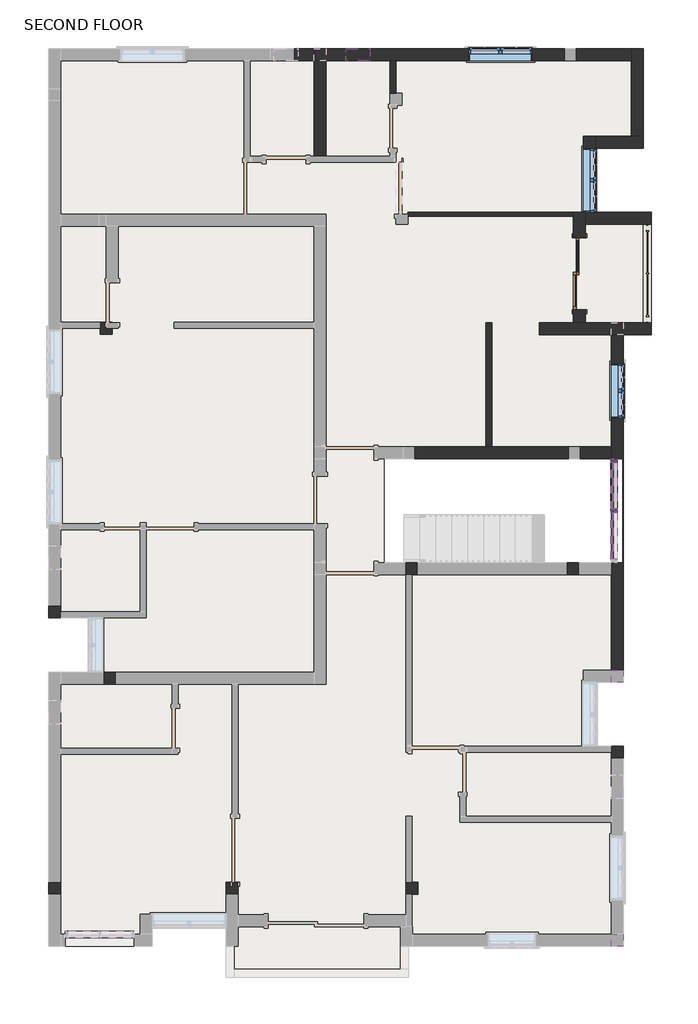
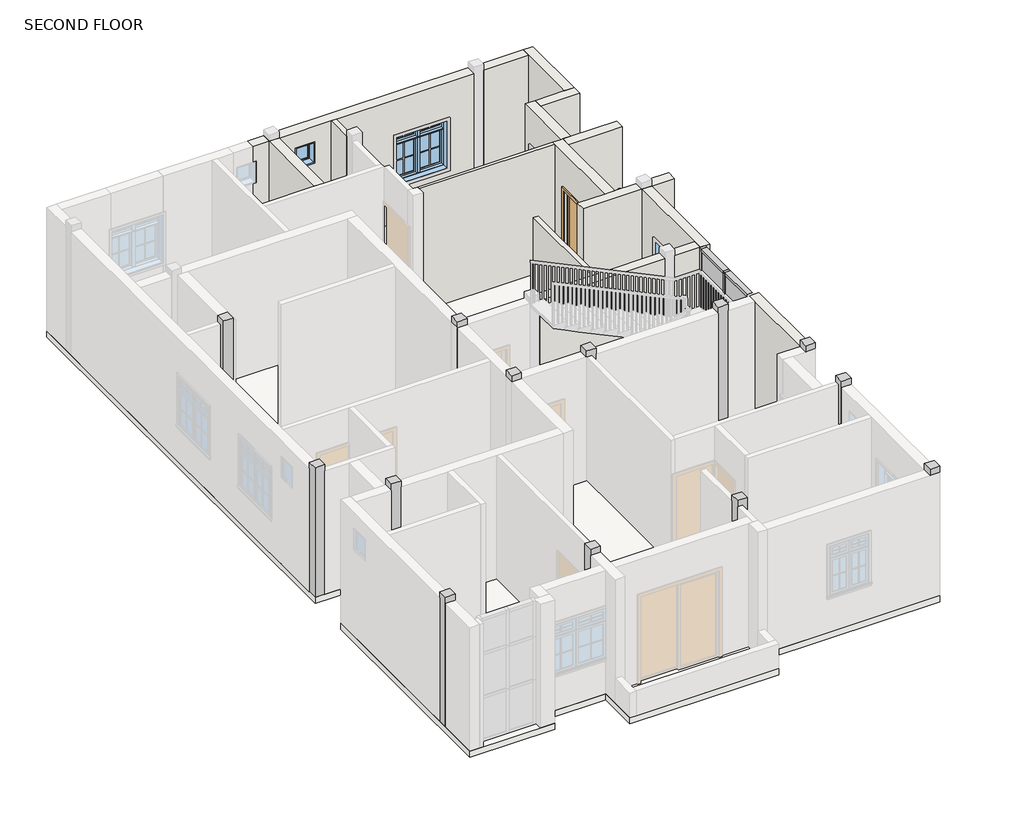
# One storey, part 3 of 6: 17 walls, 13 columns, 9 members, 4 plates, 4 windows, 1 door, 1 slab.
"""IFC4 building model written with IfcOpenShell, lengths in millimetres."""

from ifc_helpers import new_model, si_unit, frame, origin, place, context, project, spatial, polyline, outline, extrude, faceted_brep, transform, mapped, element, save
from components import door_double_sliding_4_5_x7_60868813, member_f1f71bde, member_e0487b50, member_aafbdc53, member_00c01c4d, member_0131f3aa, member_ecafcbb3, system_panel_glazed_149319f3, system_panel_glazed_118543cb, window_abb441dd, window_35f3c129, window_casement_double_awning_double_4_x4_dd9041c6

model = new_model("IFC4")

# Units and contexts
model_context = context("Model", 3, world=origin())
ifc_project = project(units=[si_unit("LENGTHUNIT", "METRE", prefix="MILLI")], contexts=[model_context])

# Site, building, storey
site = spatial("IfcSite", under=ifc_project)
building = spatial("IfcBuilding", under=site)
storey = spatial("IfcBuildingStorey", under=building, Name="SECOND FLOOR", Elevation=6400.8)

# Columns
placement = place(None, origin())
element("IfcColumn", 1, ObjectType="Rectangular Column : 9\"X9\"", at=placement, inside=storey, context=model_context, shape_type="Brep", body=[
    faceted_brep([(-5558.0284021, 3851.8787587, 6400.8), (-5786.6284021, 3851.8787587, 6400.8), (-5786.6284021, 3966.1787587, 6400.8), (-5786.6284021, 4080.4787587, 6400.8), (-5558.0284021, 4080.4787587, 6400.8), (-5558.0284021, 4074.1287587, 6400.8), (-5663.5865981, 4074.1287587, 6400.8), (-5663.5865981, 3966.1787587, 6400.8), (-5558.0284021, 3966.1787587, 6400.8), (-5558.0284021, 4080.4787587, 9601.2), (-5558.0284021, 3851.8787587, 9601.2), (-5558.0284021, 3966.1787587, 9448.8), (-5558.0284021, 4080.4787587, 9448.8), (-5786.6284021, 3851.8787587, 9601.2), (-5786.6284021, 4080.4787587, 9601.2), (-5786.6284021, 4080.4787587, 9448.8), (-5663.5865981, 4080.4787587, 9448.8), (-5663.5865981, 4080.4787587, 8534.4), (-5558.0284021, 4080.4787587, 8534.4), (-5663.5865981, 3966.1787587, 9448.8), (-5663.5865981, 4074.1287587, 8534.4), (-5558.0284021, 4074.1287587, 8534.4)], [[[0, 1, 2, 3, 4, 5, 6, 7, 8]], [[9, 10, 0, 8, 11, 12]], [[1, 0, 10, 13]], [[3, 2, 1, 13, 14, 15]], [[4, 3, 15, 14, 9, 12, 16, 17, 18]], [[10, 9, 14, 13]], [[7, 19, 11, 8]], [[19, 16, 12, 11]], [[17, 20, 21, 18]], [[20, 6, 5, 21]], [[19, 7, 6, 20, 17, 16]], [[5, 4, 18, 21]]]),
])
element("IfcColumn", 2, ObjectType="Rectangular Column : 9\"X9\"", at=placement, inside=storey, context=model_context, shape_type="Brep", body=[
    faceted_brep([(-5488.7582398, -2599.7212413, 6400.8), (-5488.7582398, -2828.3212413, 6400.8), (-5717.3582398, -2828.3212413, 6400.8), (-5717.3582398, -2599.7212413, 6400.8), (-5488.7582398, -2599.7212413, 9601.2), (-5488.7582398, -2828.3212413, 9601.2), (-5488.7582398, -2828.3212413, 9448.8), (-5488.7582398, -2599.7212413, 9448.8), (-5717.3582398, -2828.3212413, 9601.2), (-5717.3582398, -2828.3212413, 9448.8), (-5717.3582398, -2599.7212413, 9601.2), (-5717.3582398, -2599.7212413, 9448.8)], [[[0, 1, 2, 3]], [[4, 5, 6, 1, 0, 7]], [[5, 8, 9, 2, 1, 6]], [[8, 10, 11, 3, 2, 9]], [[10, 4, 7, 0, 3, 11]], [[4, 10, 8, 5]]]),
])
element("IfcColumn", 3, ObjectType="Rectangular Column : 9\"X9\"", at=placement, inside=storey, context=model_context, shape_type="Brep", body=[
    faceted_brep([(-6539.8865981, -6601.1424416, 6400.8), (-6539.8865981, -6829.7424416, 6400.8), (-6768.4865981, -6829.7424416, 6400.8), (-6768.4865981, -6601.1424416, 6400.8), (-6539.8865981, -6601.1424416, 9601.2), (-6539.8865981, -6829.7424416, 9601.2), (-6539.8865981, -6829.7424416, 9448.8), (-6539.8865981, -6601.1424416, 9448.8), (-6768.4865981, -6829.7424416, 9601.2), (-6768.4865981, -6829.7424416, 9448.8), (-6768.4865981, -6601.1424416, 9601.2), (-6768.4865981, -6601.1424416, 9448.8)], [[[0, 1, 2, 3]], [[4, 5, 6, 1, 0, 7]], [[5, 8, 9, 2, 1, 6]], [[8, 10, 11, 3, 2, 9]], [[10, 4, 7, 0, 3, 11]], [[4, 10, 8, 5]]]),
])
element("IfcColumn", 4, ObjectType="Rectangular Column : 9\"X9\"", at=placement, inside=storey, context=model_context, shape_type="Brep", body=[
    faceted_brep([(-3148.9865981, -6600.2212413, 6400.8), (-3148.9865981, -6828.8212413, 6400.8), (-3377.5865981, -6828.8212413, 6400.8), (-3377.5865981, -6600.2212413, 6400.8), (-3148.9865981, -6600.2212413, 9601.2), (-3148.9865981, -6828.8212413, 9601.2), (-3148.9865981, -6828.8212413, 9448.8), (-3148.9865981, -6600.2212413, 8534.4), (-3148.9865981, -6600.2212413, 9448.8), (-3377.5865981, -6828.8212413, 9601.2), (-3377.5865981, -6828.8212413, 9448.8), (-3377.5865981, -6600.2212413, 9601.2)], [[[0, 1, 2, 3]], [[4, 5, 6, 1, 0, 7, 8]], [[5, 9, 10, 2, 1, 6]], [[9, 11, 3, 2, 10]], [[11, 4, 8, 7, 0, 3]], [[4, 11, 9, 5]]]),
])
element("IfcColumn", 5, ObjectType="Rectangular Column : 9\"X9\"", at=placement, inside=storey, context=model_context, shape_type="Brep", body=[
    faceted_brep([(280.0134019, -6601.1424416, 6400.8), (280.0134019, -6829.7424416, 6400.8), (165.7134019, -6829.7424416, 6400.8), (51.4134019, -6829.7424416, 6400.8), (51.4134019, -6601.1424416, 6400.8), (165.7134019, -6601.1424416, 6400.8), (280.0134019, -6601.1424416, 9601.2), (280.0134019, -6829.7424416, 9601.2), (51.4134019, -6829.7424416, 9601.2), (51.4134019, -6829.7424416, 9448.8), (51.4134019, -6601.1424416, 9601.2), (51.4134019, -6601.1424416, 9448.8)], [[[0, 1, 2, 3, 4, 5]], [[6, 7, 1, 0]], [[7, 8, 9, 3, 2, 1]], [[8, 10, 11, 4, 3, 9]], [[10, 6, 0, 5, 4, 11]], [[6, 10, 8, 7]]]),
])
element("IfcColumn", 6, ObjectType="Rectangular Column : 9\"X9\"", at=placement, inside=storey, context=model_context, shape_type="SweptSolid", body=[
    extrude(outline(polyline([(4204.3134019, -7590.8212413), (4204.3134019, -7819.4212413), (3975.7134019, -7819.4212413), (3975.7134019, -7590.8212413), (4204.3134019, -7590.8212413)])), frame((0.0, 0.0, 9448.8), z_axis=(0.0, 0.0, 1.0), x_axis=(1.0, 0.0, 0.0)), (0.0, 0.0, 1.0), 152.4),
])
element("IfcColumn", 7, ObjectType="Rectangular Column : 9\"X9\"", at=placement, inside=storey, context=model_context, shape_type="Brep", body=[
    faceted_brep([(4204.3134019, -4009.4212413, 6400.8), (4204.3134019, -4238.0212413, 6400.8), (3975.7134019, -4238.0212413, 6400.8), (3975.7134019, -4123.7212413, 6400.8), (3975.7134019, -4009.4212413, 6400.8), (4204.3134019, -4009.4212413, 9601.2), (4204.3134019, -4238.0212413, 9601.2), (4204.3134019, -4238.0212413, 9448.8), (3975.7134019, -4238.0212413, 9601.2), (3975.7134019, -4238.0212413, 9448.8), (3975.7134019, -4009.4212413, 9601.2), (3975.7134019, -4009.4212413, 9448.8)], [[[0, 1, 2, 3, 4]], [[5, 6, 7, 1, 0]], [[6, 8, 9, 2, 1, 7]], [[8, 10, 11, 4, 3, 2, 9]], [[10, 5, 0, 4, 11]], [[5, 10, 8, 6]]]),
])
element("IfcColumn", 8, ObjectType="Rectangular Column : 9\"X9\"", at=placement, inside=storey, context=model_context, shape_type="Brep", body=[
    faceted_brep([(3352.7127672, -504.2212413, 6400.8), (3352.7127672, -732.8212413, 6400.8), (3124.1127672, -732.8212413, 6400.8), (3124.1127672, -504.2212413, 6400.8), (3352.7127672, -504.2212413, 9601.2), (3352.7127672, -732.8212413, 9601.2), (3352.7127672, -732.8212413, 9448.8), (3352.7127672, -504.2212413, 9448.8), (3124.1127672, -732.8212413, 9601.2), (3124.1127672, -732.8212413, 9448.8), (3124.1127672, -504.2212413, 9601.2), (3124.1127672, -504.2212413, 9448.8)], [[[0, 1, 2, 3]], [[4, 5, 6, 1, 0, 7]], [[5, 8, 9, 2, 1, 6]], [[8, 10, 11, 3, 2, 9]], [[10, 4, 7, 0, 3, 11]], [[4, 10, 8, 5]]]),
])
element("IfcColumn", 9, ObjectType="Rectangular Column : 9\"X9\"", at=placement, inside=storey, context=model_context, shape_type="Brep", body=[
    faceted_brep([(269.7035962, -504.2212413, 6400.8), (269.7035962, -732.8212413, 6400.8), (165.7134019, -732.8212413, 6400.8), (51.4134019, -732.8212413, 6400.8), (41.1035962, -732.8212413, 6400.8), (41.1035962, -504.2212413, 6400.8), (269.7035962, -504.2212413, 9601.2), (269.7035962, -732.8212413, 9601.2), (269.7035962, -732.8212413, 9448.8), (269.7035962, -504.2212413, 9448.8), (41.1035962, -732.8212413, 9601.2), (41.1035962, -732.8212413, 9448.8), (41.1035962, -504.2212413, 9601.2), (41.1035962, -504.2212413, 9448.8)], [[[0, 1, 2, 3, 4, 5]], [[6, 7, 8, 1, 0, 9]], [[7, 10, 11, 4, 3, 2, 1, 8]], [[10, 12, 13, 5, 4, 11]], [[12, 6, 9, 0, 5, 13]], [[6, 12, 10, 7]]]),
])
element("IfcColumn", 10, ObjectType="Rectangular Column : 9\"X9\"", at=placement, inside=storey, context=model_context, shape_type="Brep", body=[
    faceted_brep([(-1472.5865981, -733.7424416, 6400.8), (-1701.1865981, -733.7424416, 6400.8), (-1701.1865981, -732.8212413, 6400.8), (-1472.5865981, -732.8212413, 6400.8), (-1472.5865981, -505.1424416, 9601.2), (-1472.5865981, -733.7424416, 9601.2), (-1472.5865981, -733.7424416, 9448.8), (-1472.5865981, -732.8212413, 8534.4), (-1472.5865981, -732.8212413, 9448.8), (-1472.5865981, -505.1424416, 9448.8), (-1701.1865981, -733.7424416, 9601.2), (-1701.1865981, -733.7424416, 9448.8), (-1701.1865981, -505.1424416, 9601.2), (-1701.1865981, -505.1424416, 9448.8), (-1701.1865981, -732.8212413, 9448.8)], [[[0, 1, 2, 3]], [[4, 5, 6, 0, 3, 7, 8, 9]], [[1, 0, 6, 5, 10, 11]], [[1, 11, 10, 12, 13, 14, 2]], [[12, 4, 9, 13]], [[5, 4, 12, 10]], [[14, 8, 7, 3, 2]], [[8, 14, 13, 9]]]),
])
element("IfcColumn", 11, ObjectType="Rectangular Column : 9\"X9\"", at=placement, inside=storey, context=model_context, shape_type="Brep", body=[
    faceted_brep([(-1472.5865981, 1464.4966521, 6400.8), (-1701.1865981, 1464.4966521, 6400.8), (-1701.1865981, 1476.9787587, 6400.8), (-1472.5865981, 1476.9787587, 6400.8), (-1472.5865981, 1693.0966521, 9601.2), (-1472.5865981, 1464.4966521, 9601.2), (-1472.5865981, 1464.4966521, 9448.8), (-1472.5865981, 1476.9787587, 8534.4), (-1472.5865981, 1476.9787587, 9448.8), (-1472.5865981, 1693.0966521, 9448.8), (-1701.1865981, 1464.4966521, 9601.2), (-1701.1865981, 1464.4966521, 9448.8), (-1701.1865981, 1693.0966521, 9601.2), (-1701.1865981, 1693.0966521, 9448.8), (-1701.1865981, 1476.9787587, 9448.8)], [[[0, 1, 2, 3]], [[4, 5, 6, 0, 3, 7, 8, 9]], [[1, 0, 6, 5, 10, 11]], [[1, 11, 10, 12, 13, 14, 2]], [[12, 4, 9, 13]], [[5, 4, 12, 10]], [[14, 8, 7, 3, 2]], [[8, 14, 13, 9]]]),
])
element("IfcColumn", 12, ObjectType="Rectangular Column : 9\"X9\"", at=placement, inside=storey, context=model_context, shape_type="Brep", body=[
    faceted_brep([(-6539.8865981, -1329.7212413, 6400.8), (-6539.8865981, -1444.0212413, 6400.8), (-6539.8865981, -1558.3212413, 6400.8), (-6768.4865981, -1558.3212413, 6400.8), (-6768.4865981, -1329.7212413, 6400.8), (-6539.8865981, -1329.7212413, 9601.2), (-6539.8865981, -1558.3212413, 9601.2), (-6539.8865981, -1558.3212413, 9448.8), (-6539.8865981, -1329.7212413, 9448.8), (-6768.4865981, -1558.3212413, 9601.2), (-6768.4865981, -1329.7212413, 9601.2), (-6768.4865981, -1329.7212413, 9448.8)], [[[0, 1, 2, 3, 4]], [[5, 6, 7, 2, 1, 0, 8]], [[6, 9, 3, 2, 7]], [[9, 10, 11, 4, 3]], [[10, 5, 8, 0, 4, 11]], [[5, 10, 9, 6]]]),
])
element("IfcColumn", 13, ObjectType="Rectangular Column : 9\"X9\"", at=placement, inside=storey, context=model_context, shape_type="SweptSolid", body=[
    extrude(outline(polyline([(4204.3134019, -2561.6212413), (4204.3134019, -2790.2212413), (3975.7134019, -2790.2212413), (3975.7134019, -2561.6212413), (4204.3134019, -2561.6212413)])), frame((0.0, 0.0, 9448.8), z_axis=(0.0, 0.0, 1.0), x_axis=(1.0, 0.0, 0.0)), (0.0, 0.0, 1.0), 152.4),
])

# Door
door_double_sliding_4_5_x7_shape = door_double_sliding_4_5_x7_60868813(model_context)
element("IfcDoor", 14, ObjectType="Door-Double-Sliding : 4.5'X7'", at=placement, inside=storey, context=model_context, shape_type="MappedRepresentation", body=[
    mapped(door_double_sliding_4_5_x7_shape, transform((3493.1134019, 5007.5787587, 6400.8), x_axis=(0.0, 1.0, 0.0), y_axis=(-1.0, 0.0, 0.0), z_axis=(0.0, 0.0, 1.0))),
])

# Members
member_shape = member_f1f71bde(model_context)
element("IfcMember", 15, ObjectType="Rectangular Mullion : 2.5\" x 5\" rectangular", at=placement, inside=storey, context=model_context, shape_type="MappedRepresentation", body=[
    mapped(member_shape, transform((4026.5134019, 1413.4787587, 9448.8), x_axis=(0.0, 0.0, 1.0), y_axis=(1.0, 0.0, 0.0), z_axis=(0.0, 1.0, 0.0))),
])
element("IfcMember", 16, ObjectType="Rectangular Mullion : 2.5\" x 5\" rectangular", at=placement, inside=storey, context=model_context, shape_type="MappedRepresentation", body=[
    mapped(member_shape, transform((4026.5134019, 454.6287587, 9448.8), x_axis=(0.0, 0.0, 1.0), y_axis=(1.0, 0.0, 0.0), z_axis=(0.0, 1.0, 0.0))),
])
element("IfcMember", 17, ObjectType="Rectangular Mullion : 2.5\" x 5\" rectangular", at=placement, inside=storey, context=model_context, shape_type="MappedRepresentation", body=[
    mapped(member_shape, transform((4026.5134019, 518.1287587, 6400.8), x_axis=(0.0, 0.0, -1.0), y_axis=(1.0, 0.0, 0.0), z_axis=(0.0, -1.0, 0.0))),
])
member_2_shape = member_e0487b50(model_context)
element("IfcMember", 18, ObjectType="Rectangular Mullion : 2.5\" x 5\" rectangular", at=placement, inside=storey, context=model_context, shape_type="MappedRepresentation", body=[
    mapped(member_2_shape, transform((4026.5134019, 454.6287587, 7956.55), x_axis=(0.0, 0.0, 1.0), y_axis=(1.0, 0.0, 0.0), z_axis=(0.0, 1.0, 0.0))),
])
element("IfcMember", 19, ObjectType="Rectangular Mullion : 2.5\" x 5\" rectangular", at=placement, inside=storey, context=model_context, shape_type="MappedRepresentation", body=[
    mapped(member_2_shape, transform((4026.5134019, 1413.4787587, 7956.55), x_axis=(0.0, 0.0, 1.0), y_axis=(1.0, 0.0, 0.0), z_axis=(0.0, 1.0, 0.0))),
])
member_3_shape = member_aafbdc53(model_context)
element("IfcMember", 20, ObjectType="Rectangular Mullion : 2.5\" x 5\" rectangular", at=placement, inside=storey, context=model_context, shape_type="MappedRepresentation", body=[
    mapped(member_3_shape, transform((4026.5134019, 486.3787587, 6400.8), x_axis=(0.0, 1.0, 0.0), y_axis=(1.0, 0.0, 0.0), z_axis=(0.0, 0.0, -1.0))),
])
member_4_shape = member_00c01c4d(model_context)
element("IfcMember", 21, ObjectType="Rectangular Mullion : 2.5\" x 5\" rectangular", at=placement, inside=storey, context=model_context, shape_type="MappedRepresentation", body=[
    mapped(member_4_shape, transform((4026.5134019, 1476.9787587, 6400.8), x_axis=(0.0, 1.0, 0.0), y_axis=(1.0, 0.0, 0.0), z_axis=(0.0, 0.0, -1.0))),
])
member_5_shape = member_0131f3aa(model_context)
element("IfcMember", 22, ObjectType="Rectangular Mullion : 2.5\" x 5\" rectangular", at=placement, inside=storey, context=model_context, shape_type="MappedRepresentation", body=[
    mapped(member_5_shape, transform((4026.5134019, 486.3787587, 7956.55), x_axis=(0.0, 1.0, 0.0), y_axis=(1.0, 0.0, 0.0), z_axis=(0.0, 0.0, -1.0))),
])
member_6_shape = member_ecafcbb3(model_context)
element("IfcMember", 23, ObjectType="Rectangular Mullion : 2.5\" x 5\" rectangular", at=placement, inside=storey, context=model_context, shape_type="MappedRepresentation", body=[
    mapped(member_6_shape, transform((4026.5134019, 1476.9787587, 7956.55), x_axis=(0.0, 1.0, 0.0), y_axis=(1.0, 0.0, 0.0), z_axis=(0.0, 0.0, -1.0))),
])

# Plates
system_panel_glazed_shape = system_panel_glazed_149319f3(model_context)
element("IfcPlate", 24, ObjectType="System Panel : Glazed", at=placement, inside=storey, context=model_context, shape_type="MappedRepresentation", body=[
    mapped(system_panel_glazed_shape, transform((4026.5134019, 6.9537587, 6464.3), x_axis=(0.0, 1.0, 0.0), y_axis=(-1.0, 0.0, 0.0), z_axis=(0.0, 0.0, 1.0))),
])
element("IfcPlate", 25, ObjectType="System Panel : Glazed", at=placement, inside=storey, context=model_context, shape_type="MappedRepresentation", body=[
    mapped(system_panel_glazed_shape, transform((4026.5134019, 965.8037587, 6464.3), x_axis=(0.0, 1.0, 0.0), y_axis=(-1.0, 0.0, 0.0), z_axis=(0.0, 0.0, 1.0))),
])
system_panel_glazed_2_shape = system_panel_glazed_118543cb(model_context)
element("IfcPlate", 26, ObjectType="System Panel : Glazed", at=placement, inside=storey, context=model_context, shape_type="MappedRepresentation", body=[
    mapped(system_panel_glazed_2_shape, transform((4026.5134019, 6.9537587, 7988.3), x_axis=(0.0, 1.0, 0.0), y_axis=(-1.0, 0.0, 0.0), z_axis=(0.0, 0.0, 1.0))),
])
element("IfcPlate", 27, ObjectType="System Panel : Glazed", at=placement, inside=storey, context=model_context, shape_type="MappedRepresentation", body=[
    mapped(system_panel_glazed_2_shape, transform((4026.5134019, 965.8037587, 7988.3), x_axis=(0.0, 1.0, 0.0), y_axis=(-1.0, 0.0, 0.0), z_axis=(0.0, 0.0, 1.0))),
])

# Slab
element("IfcSlab", 28, ObjectType="6\"", at=placement, inside=storey, context=model_context, shape_type="SweptSolid", body=[
    extrude(outline(polyline([(-6768.4865981, -1558.3212413), (-6768.4865981, 9300.1787587), (4585.3134019, 9300.1787587), (4585.3134019, 7395.1787587), (3670.9134019, 7395.1787587), (3670.9134019, 6175.9787587), (4737.7134019, 6175.9787587), (4737.7134019, 3839.1787587), (4204.3134019, 3839.1787587), (4204.3134019, -2790.2212413), (3670.9134019, -2790.2212413), (3670.9134019, -4009.4212413), (4204.3134019, -4009.4212413), (4204.3134019, -7819.4212413), (102.2134019, -7819.4212413), (102.2134019, -8416.3212413), (-3377.5865981, -8416.3212413), (-3377.5865981, -7438.4212413), (-4787.2865981, -7438.4212413), (-4787.2865981, -7819.4212413), (-6768.4865981, -7819.4212413), (-6768.4865981, -2599.7212413), (-5974.2886947, -2599.7212413), (-5974.2886947, -1558.3212413), (-6768.4865981, -1558.3212413)]), holes=[polyline([(4178.9134019, 1705.5787587), (-353.2951421, 1705.5787587), (-353.2951421, -732.8212413), (4178.9134019, -732.8212413), (4178.9134019, 1705.5787587)])]), frame((0.0, 0.0, 6248.4), z_axis=(0.0, 0.0, 1.0), x_axis=(1.0, 0.0, 0.0)), (0.0, 0.0, 1.0), 152.4),
])

# Walls
element("IfcWall", 29, ObjectType="3\"", at=placement, inside=storey, context=model_context, shape_type="Brep", body=[
    faceted_brep([(3251.8134019, 6175.9787587, 6400.8), (89.5134019, 6175.9787587, 6400.8), (89.5134019, 6175.9787587, 8534.4), (89.5134019, 6175.9787587, 9448.8), (3251.8134019, 6175.9787587, 9448.8), (3251.8134019, 6099.7787587, 6400.8), (3251.8134019, 6099.7787587, 9448.8), (89.5134019, 6099.7787587, 9448.8), (89.5134019, 6099.7787587, 6400.8), (89.5134019, 6137.8787587, 6400.8)], [[[0, 1, 2, 3, 4]], [[5, 6, 7, 8]], [[1, 0, 5, 8, 9]], [[4, 3, 7, 6]], [[0, 4, 6, 5]], [[3, 2, 1, 9, 8, 7]]]),
])
element("IfcWall", 30, ObjectType="4.5\"", at=placement, inside=storey, context=model_context, shape_type="SweptSolid", body=[
    extrude(outline(polyline([(-139.0865981, 9071.5787587), (-139.0865981, 8443.0921256), (-253.3865981, 8443.0921256), (-253.3865981, 9071.5787587), (-139.0865981, 9071.5787587)])), frame((0.0, 0.0, 6400.8), z_axis=(0.0, 0.0, 1.0), x_axis=(1.0, 0.0, 0.0)), (0.0, 0.0, 1.0), 3048.0),
])
element("IfcWall", 31, ObjectType="4.5\"", at=placement, inside=storey, context=model_context, shape_type="SweptSolid", body=[
    extrude(outline(polyline([(1575.4134019, 1705.5787587), (1575.4134019, 4067.7787587), (1689.7134019, 4067.7787587), (1689.7134019, 1705.5787587), (1575.4134019, 1705.5787587)])), frame((0.0, 0.0, 6400.8), z_axis=(0.0, 0.0, 1.0), x_axis=(1.0, 0.0, 0.0)), (0.0, 0.0, 1.0), 3048.0),
])
element("IfcWall", 32, ObjectType="6\"", at=placement, inside=storey, context=model_context, shape_type="SweptSolid", body=[
    extrude(outline(polyline([(4585.3134019, 4067.7787587), (4585.3134019, 5947.3787587), (4737.7134019, 5947.3787587), (4737.7134019, 4067.7787587), (4585.3134019, 4067.7787587)])), frame((0.0, 0.0, 6400.8), z_axis=(0.0, 0.0, 1.0), x_axis=(1.0, 0.0, 0.0)), (0.0, 0.0, 1.0), 609.6),
])
element("IfcWall", 33, ObjectType="9\"", at=placement, inside=storey, context=model_context, shape_type="Brep", body=[
    faceted_brep([(4204.3134019, -2561.6212413, 9448.8), (4204.3134019, -2561.6212413, 6400.8), (4204.3134019, -504.2212413, 6400.8), (4204.3134019, -504.2212413, 9448.8), (3975.7134019, -2561.6212413, 6400.8), (3975.7134019, -2561.6212413, 9448.8), (3975.7134019, -732.8212413, 9448.8), (3975.7134019, -504.2212413, 9448.8), (3975.7134019, -504.2212413, 6400.8), (3975.7134019, -732.8212413, 6400.8)], [[[0, 1, 2, 3]], [[4, 5, 6, 7, 8, 9]], [[1, 4, 9, 8, 2]], [[5, 0, 3, 7, 6]], [[1, 0, 5, 4]], [[3, 2, 8, 7]]]),
    faceted_brep([(4204.3134019, 3839.1787587, 6400.8), (4204.3134019, 3839.1787587, 9448.8), (4204.3134019, 1476.9787587, 9448.8), (4204.3134019, 1476.9787587, 6400.8), (4204.3134019, 2251.6787587, 7315.2), (4204.3134019, 2251.6787587, 8534.4), (4204.3134019, 3293.0787587, 8534.4), (4204.3134019, 3293.0787587, 7315.2), (3975.7134019, 3839.1787587, 9448.8), (3975.7134019, 3839.1787587, 6400.8), (3975.7134019, 1705.5787587, 6400.8), (3975.7134019, 1476.9787587, 6400.8), (3975.7134019, 1476.9787587, 9448.8), (3975.7134019, 1705.5787587, 9448.8), (3975.7134019, 2251.6787587, 8534.4), (3975.7134019, 2251.6787587, 7315.2), (3975.7134019, 3293.0787587, 7315.2), (3975.7134019, 3293.0787587, 8534.4)], [[[0, 1, 2, 3], [4, 5, 6, 7]], [[8, 9, 10, 11, 12, 13], [14, 15, 16, 17]], [[9, 0, 3, 11, 10]], [[1, 8, 13, 12, 2]], [[1, 0, 9, 8]], [[15, 14, 5, 4]], [[16, 15, 4, 7]], [[17, 16, 7, 6]], [[14, 17, 6, 5]], [[3, 2, 12, 11]]]),
])
element("IfcWall", 34, ObjectType="9\"", at=placement, inside=storey, context=model_context, shape_type="Brep", body=[
    faceted_brep([(229.251657, 1476.9787587, 6400.8), (3156.5070369, 1476.9787587, 6400.8), (3156.5070369, 1476.9787587, 9448.8), (229.251657, 1476.9787587, 9448.8), (229.251657, 1705.5787587, 6400.8), (229.251657, 1705.5787587, 9448.8), (1575.4134019, 1705.5787587, 9448.8), (1689.7134019, 1705.5787587, 9448.8), (3156.5070369, 1705.5787587, 9448.8), (3156.5070369, 1705.5787587, 6400.8), (1689.7134019, 1705.5787587, 6400.8), (1575.4134019, 1705.5787587, 6400.8)], [[[0, 1, 2, 3]], [[4, 5, 6, 7, 8, 9, 10, 11]], [[1, 0, 4, 11, 10, 9]], [[2, 1, 9, 8]], [[3, 2, 8, 7, 6, 5]], [[0, 3, 5, 4]]]),
])
element("IfcWall", 35, ObjectType="9\"", at=placement, inside=storey, context=model_context, shape_type="SweptSolid", body=[
    extrude(outline(polyline([(3975.7134019, 1476.9787587), (3385.1070369, 1476.9787587), (3385.1070369, 1705.5787587), (3975.7134019, 1705.5787587), (3975.7134019, 1476.9787587)])), frame((0.0, 0.0, 6400.8), z_axis=(0.0, 0.0, 1.0), x_axis=(1.0, 0.0, 0.0)), (0.0, 0.0, 1.0), 3048.0),
])
element("IfcWall", 36, ObjectType="9\"", at=placement, inside=storey, context=model_context, shape_type="Brep", body=[
    faceted_brep([(2604.1134019, 3839.1787587, 6400.8), (3975.7134019, 3839.1787587, 6400.8), (4204.3134019, 3839.1787587, 6400.8), (4737.7134019, 3839.1787587, 6400.8), (4737.7134019, 3839.1787587, 9448.8), (4204.3134019, 3839.1787587, 9448.8), (3975.7134019, 3839.1787587, 9448.8), (2604.1134019, 3839.1787587, 9448.8), (2604.1134019, 4067.7787587, 6400.8), (2604.1134019, 4067.7787587, 9448.8), (3251.8134019, 4067.7787587, 9448.8), (3480.4134019, 4067.7787587, 9448.8), (3975.7134019, 4067.7787587, 9448.8), (4204.3134019, 4067.7787587, 9448.8), (4737.7134019, 4067.7787587, 9448.8), (4737.7134019, 4067.7787587, 7010.4), (4737.7134019, 4067.7787587, 6400.8), (4585.3134019, 4067.7787587, 6400.8), (3480.4134019, 4067.7787587, 6400.8), (3251.8134019, 4067.7787587, 6400.8)], [[[0, 1, 2, 3, 4, 5, 6, 7]], [[8, 9, 10, 11, 12, 13, 14, 15, 16, 17, 18, 19]], [[3, 2, 1, 0, 8, 19, 18, 17, 16]], [[7, 6, 5, 4, 14, 13, 12, 11, 10, 9]], [[0, 7, 9, 8]], [[4, 3, 16, 15, 14]]]),
])
element("IfcWall", 37, ObjectType="9\"", at=placement, inside=storey, context=model_context, shape_type="Brep", body=[
    faceted_brep([(3480.4134019, 5693.3787587, 8534.4), (3480.4134019, 5693.3787587, 6400.8), (3480.4134019, 5947.3787587, 6400.8), (3480.4134019, 6175.9787587, 6400.8), (3480.4134019, 6175.9787587, 9448.8), (3480.4134019, 5947.3787587, 9448.8), (3480.4134019, 4067.7787587, 9448.8), (3480.4134019, 4067.7787587, 6400.8), (3480.4134019, 4321.7787587, 6400.8), (3480.4134019, 4321.7787587, 8534.4), (3251.8134019, 6175.9787587, 6400.8), (3251.8134019, 6099.7787587, 6400.8), (3251.8134019, 5693.3787587, 6400.8), (3251.8134019, 5693.3787587, 8534.4), (3251.8134019, 4321.7787587, 8534.4), (3251.8134019, 4321.7787587, 6400.8), (3251.8134019, 4067.7787587, 6400.8), (3251.8134019, 4067.7787587, 9448.8), (3251.8134019, 6099.7787587, 9448.8), (3251.8134019, 6175.9787587, 9448.8), (3442.3134019, 6175.9787587, 6400.8), (3442.3134019, 6175.9787587, 9448.8)], [[[0, 1, 2, 3, 4, 5, 6, 7, 8, 9]], [[10, 11, 12, 13, 14, 15, 16, 17, 18, 19]], [[8, 7, 16, 15]], [[3, 2, 1, 12, 11, 10, 20]], [[6, 5, 4, 21, 19, 18, 17]], [[7, 6, 17, 16]], [[4, 3, 20, 10, 19, 21]], [[15, 14, 9, 8]], [[13, 12, 1, 0]], [[14, 13, 0, 9]]]),
])
element("IfcWall", 38, ObjectType="9\"", at=placement, inside=storey, context=model_context, shape_type="Brep", body=[
    faceted_brep([(3480.4134019, 5947.3787587, 6400.8), (4585.3134019, 5947.3787587, 6400.8), (4737.7134019, 5947.3787587, 6400.8), (4737.7134019, 5947.3787587, 7010.4), (4737.7134019, 5947.3787587, 9448.8), (3480.4134019, 5947.3787587, 9448.8), (3480.4134019, 6175.9787587, 6400.8), (3480.4134019, 6175.9787587, 9448.8), (3670.9134019, 6175.9787587, 9448.8), (4737.7134019, 6175.9787587, 9448.8), (4737.7134019, 6175.9787587, 6400.8), (3670.9134019, 6175.9787587, 6400.8)], [[[0, 1, 2, 3, 4, 5]], [[6, 7, 8, 9, 10, 11]], [[2, 1, 0, 6, 11, 10]], [[5, 4, 9, 8, 7]], [[0, 5, 7, 6]], [[4, 3, 2, 10, 9]]]),
])
element("IfcWall", 39, ObjectType="9\"", at=placement, inside=storey, context=model_context, shape_type="Brep", body=[
    faceted_brep([(3670.9134019, 7395.1787587, 7315.2), (3670.9134019, 6175.9787587, 7315.2), (3670.9134019, 6175.9787587, 6400.8), (3670.9134019, 7395.1787587, 6400.8), (3670.9134019, 7623.7787587, 6400.8), (3670.9134019, 7623.7787587, 9448.8), (3670.9134019, 7395.1787587, 9448.8), (3670.9134019, 6175.9787587, 9448.8), (3670.9134019, 6175.9787587, 8534.4), (3670.9134019, 7395.1787587, 8534.4), (3442.3134019, 6175.9787587, 6400.8), (3442.3134019, 6175.9787587, 7315.2), (3442.3134019, 7395.1787587, 7315.2), (3442.3134019, 7395.1787587, 8534.4), (3442.3134019, 6175.9787587, 8534.4), (3442.3134019, 6175.9787587, 9448.8), (3442.3134019, 7623.7787587, 9448.8), (3442.3134019, 7623.7787587, 6400.8), (3480.4134019, 6175.9787587, 6400.8), (3480.4134019, 6175.9787587, 9448.8)], [[[0, 1, 2, 3, 4, 5, 6, 7, 8, 9]], [[10, 11, 12, 13, 14, 15, 16, 17]], [[4, 3, 2, 18, 10, 17]], [[7, 6, 5, 16, 15, 19]], [[8, 7, 19, 15, 14]], [[2, 1, 11, 10, 18]], [[5, 4, 17, 16]], [[12, 11, 1, 0]], [[13, 12, 0, 9]], [[14, 13, 9, 8]]]),
])
element("IfcWall", 40, ObjectType="9\"", at=placement, inside=storey, context=model_context, shape_type="Brep", body=[
    faceted_brep([(3670.9134019, 7395.1787587, 6400.8), (4585.3134019, 7395.1787587, 6400.8), (4585.3134019, 7395.1787587, 9448.8), (3670.9134019, 7395.1787587, 9448.8), (3670.9134019, 7395.1787587, 8534.4), (3670.9134019, 7395.1787587, 7315.2), (3670.9134019, 7623.7787587, 6400.8), (3670.9134019, 7623.7787587, 9448.8), (4356.7134019, 7623.7787587, 9448.8), (4585.3134019, 7623.7787587, 9448.8), (4585.3134019, 7623.7787587, 6400.8), (4356.7134019, 7623.7787587, 6400.8)], [[[0, 1, 2, 3, 4, 5]], [[6, 7, 8, 9, 10, 11]], [[1, 0, 6, 11, 10]], [[3, 2, 9, 8, 7]], [[0, 5, 4, 3, 7, 6]], [[2, 1, 10, 9]]]),
])
element("IfcWall", 41, ObjectType="9\"", at=placement, inside=storey, context=model_context, shape_type="Brep", body=[
    faceted_brep([(4585.3134019, 7623.7787587, 6400.8), (4585.3134019, 9300.1787587, 6400.8), (4585.3134019, 9300.1787587, 9448.8), (4585.3134019, 7623.7787587, 9448.8), (4356.7134019, 7623.7787587, 6400.8), (4356.7134019, 7623.7787587, 9448.8), (4356.7134019, 9071.5787587, 9448.8), (4356.7134019, 9300.1787587, 9448.8), (4356.7134019, 9300.1787587, 6400.8), (4356.7134019, 9071.5787587, 6400.8)], [[[0, 1, 2, 3]], [[4, 5, 6, 7, 8, 9]], [[1, 0, 4, 9, 8]], [[3, 2, 7, 6, 5]], [[0, 3, 5, 4]], [[2, 1, 8, 7]]]),
])
element("IfcWall", 42, ObjectType="9\"", at=placement, inside=storey, context=model_context, shape_type="SweptSolid", body=[
    extrude(outline(polyline([(3305.8577655, 9300.1787587), (4356.7134019, 9300.1787587), (4356.7134019, 9071.5787587), (3305.8577655, 9071.5787587), (3305.8577655, 9300.1787587)])), frame((0.0, 0.0, 6400.8), z_axis=(0.0, 0.0, 1.0), x_axis=(1.0, 0.0, 0.0)), (0.0, 0.0, 1.0), 3048.0),
])
element("IfcWall", 43, ObjectType="9\"", at=placement, inside=storey, context=model_context, shape_type="Brep", body=[
    faceted_brep([(3077.2577655, 9300.1787587, 6400.8), (-1701.1865981, 9300.1787587, 6400.8), (-1701.1865981, 9300.1787587, 9448.8), (-1472.5865981, 9300.1787587, 9448.8), (3077.2577655, 9300.1787587, 9448.8), (-634.3865981, 9300.1787587, 9067.8), (-1091.5865981, 9300.1787587, 9067.8), (-1091.5865981, 9300.1787587, 8534.4), (-634.3865981, 9300.1787587, 8534.4), (2467.6577655, 9300.1787587, 8534.4), (1248.4577655, 9300.1787587, 8534.4), (1248.4577655, 9300.1787587, 7315.2), (2467.6577655, 9300.1787587, 7315.2), (3077.2577655, 9071.5787587, 6400.8), (3077.2577655, 9071.5787587, 9448.8), (-139.0865981, 9071.5787587, 9448.8), (-253.3865981, 9071.5787587, 9448.8), (-1472.5865981, 9071.5787587, 9448.8), (-1701.1865981, 9071.5787587, 9448.8), (-1701.1865981, 9071.5787587, 6400.8), (-1472.5865981, 9071.5787587, 6400.8), (-253.3865981, 9071.5787587, 6400.8), (-139.0865981, 9071.5787587, 6400.8), (-634.3865981, 9071.5787587, 9067.8), (-634.3865981, 9071.5787587, 8534.4), (-1091.5865981, 9071.5787587, 8534.4), (-1091.5865981, 9071.5787587, 9067.8), (2467.6577655, 9071.5787587, 8534.4), (2467.6577655, 9071.5787587, 7315.2), (1248.4577655, 9071.5787587, 7315.2), (1248.4577655, 9071.5787587, 8534.4)], [[[0, 1, 2, 3, 4], [5, 6, 7, 8], [9, 10, 11, 12]], [[13, 14, 15, 16, 17, 18, 19, 20, 21, 22], [23, 24, 25, 26], [27, 28, 29, 30]], [[1, 0, 13, 22, 21, 20, 19]], [[4, 3, 2, 18, 17, 16, 15, 14]], [[0, 4, 14, 13]], [[2, 1, 19, 18]], [[24, 23, 5, 8]], [[25, 24, 8, 7]], [[26, 25, 7, 6]], [[23, 26, 6, 5]], [[28, 27, 9, 12]], [[29, 28, 12, 11]], [[30, 29, 11, 10]], [[27, 30, 10, 9]]]),
])
element("IfcWall", 44, ObjectType="9\"", at=placement, inside=storey, context=model_context, shape_type="SweptSolid", body=[
    extrude(outline(polyline([(6400.8, -2082.1865981), (6400.8, -1701.1865981), (9448.8, -1701.1865981), (9448.8, -2082.1865981), (9067.8, -2082.1865981), (9067.8, -2005.9865981), (8534.4, -2005.9865981), (8534.4, -2082.1865981), (6400.8, -2082.1865981)])), frame((0.0, 9071.5787587, 0.0), z_axis=(0.0, 1.0, 0.0), x_axis=(0.0, 0.0, 1.0)), (0.0, 0.0, 1.0), 228.6),
])
element("IfcWall", 45, ObjectType="9\"", at=placement, inside=storey, context=model_context, shape_type="SweptSolid", body=[
    extrude(outline(polyline([(-1701.1865981, 7242.7787587), (-1701.1865981, 9071.5787587), (-1472.5865981, 9071.5787587), (-1472.5865981, 7242.7787587), (-1701.1865981, 7242.7787587)])), frame((0.0, 0.0, 6400.8), z_axis=(0.0, 0.0, 1.0), x_axis=(1.0, 0.0, 0.0)), (0.0, 0.0, 1.0), 3048.0),
])

# Windows
window_shape = window_abb441dd(model_context)
element("IfcWindow", 46, ObjectType="Fixed : 1'6\"X1'9\"", at=placement, inside=storey, context=model_context, shape_type="MappedRepresentation", body=[
    mapped(window_shape, transform((-824.8865981, 9185.8787587, 6400.8), x_axis=(1.0, 0.0, 0.0), y_axis=(0.0, 1.0, 0.0), z_axis=(0.0, 0.0, 1.0))),
])
window_2_shape = window_35f3c129(model_context)
element("IfcWindow", 47, ObjectType="Window-Casement-Double-Awning-Double : 3'5\"X7'", at=placement, inside=storey, context=model_context, shape_type="MappedRepresentation", body=[
    mapped(window_2_shape, transform((4090.0134019, 2772.3787587, 6400.8), x_axis=(0.0, -1.0, 0.0), y_axis=(1.0, 0.0, 0.0), z_axis=(0.0, 0.0, 1.0))),
])
window_casement_double_awning_double_4_x4_shape = window_casement_double_awning_double_4_x4_dd9041c6(model_context)
element("IfcWindow", 48, ObjectType="Window-Casement-Double-Awning-Double : 4'X4'", at=placement, inside=storey, context=model_context, shape_type="MappedRepresentation", body=[
    mapped(window_casement_double_awning_double_4_x4_shape, transform((3556.6134019, 6785.5787587, 6400.8), x_axis=(0.0, -1.0, 0.0), y_axis=(1.0, 0.0, 0.0), z_axis=(0.0, 0.0, 1.0))),
])
element("IfcWindow", 49, ObjectType="Window-Casement-Double-Awning-Double : 4'X4'", at=placement, inside=storey, context=model_context, shape_type="MappedRepresentation", body=[
    mapped(window_casement_double_awning_double_4_x4_shape, transform((1858.0577655, 9185.8787587, 6400.8), x_axis=(1.0, 0.0, 0.0), y_axis=(0.0, 1.0, 0.0), z_axis=(0.0, 0.0, 1.0))),
])

save(model, "model.ifc")

# Revit data of these elements
# Type "Rectangular Column : 9\"X9\""
#   Assembly Code = "B1010200"
#   Depth = 0' - 9"
#   Offset Base = 0' - 0"
#   Offset Top = 0' - 0"
#   Width = 0' - 9"
#   Material = none
# Type "Door-Double-Sliding : 4.5'X7'"
#   Type Mark = "14"
#   Construction Type Id = "opn-d45"
#   Assembly Code = "C1020"
#   Analytic Construction = "Wood frame, double glass door "
#   Thickness = 0' - 2"
#   Thermal Resistance (R) = 1.8150 (h·ft²·°F)/BTU
#   Heat Transfer Coefficient (U) = 0.5510 BTU/(h·ft²·°F)
#   Height = 7' - 0"
#   Rail Width = 0' - 2"
#   Stiles = 0' - 2"
#   Trim Projection Ext = 0' - 1"
#   Trim Projection Int = 0' - 1"
#   Trim Width = 0' - 3"
#   Width = 4' - 6"
#   Define Thermal Properties by = 1
#   Glazing = Glass
#   Panel Material = Wood - Birch - Solid Stained Light Low Gloss
#   Trim Material = Paint - Sienna
#   Visual Light Transmittance = 0
#   Solar Heat Gain Coefficient = 0
#   Function = (empty or 0)
#   Wall Closure = (empty or 0)
# Type "Rectangular Mullion : 2.5\" x 5\" rectangular"
#   built-in parameter 1007304 = 0.416667 (stored number, unit not read)
#   built-in parameter 1007301 = 0.104167 (stored number, unit not read)
#   built-in parameter 1007300 = 0.104167 (stored number, unit not read)
# Type "System Panel : Glazed"
#   Construction Type Id = "GSP4R"
#   Analytic Construction = "1/8 in Pilkington single glazing"
#   Visual Light Transmittance = 0.9
#   Solar Heat Gain Coefficient = 0.86
#   Heat Transfer Coefficient (U) = 1.18115 BTU/(h·ft²·°F)
#   Define Thermal Properties by = 1
# Type "6\""
#   Assembly Code = "B1010"
#   Function = 0
#   Layers, outside or top first: 0' - 6" no material (function 1)
# Type "3\""
#   Assembly Code = "B2010"
#   Layers, outside or top first: 0' - 3" no material (function 1)
# Type "4.5\""
#   Assembly Code = "B2010"
#   Layers, outside or top first: 0' - 4 1/2" no material (function 1)
# Type "6\""
#   Assembly Code = "B2010"
#   Layers, outside or top first: 0' - 6" "wood 1" (function 1)
# Type "9\""
#   Assembly Code = "B2010"
#   Layers, outside or top first: 0' - 9" "wall" (function 1)
# Type "Fixed : 1'6\"X1'9\""
#   Type Mark = "24"
#   Construction Type Id = "GSP4R"
#   Assembly Code = "B2020100"
#   Analytic Construction = "1/8 in Pilkington single glazing"
#   Visual Light Transmittance = 0.9
#   Solar Heat Gain Coefficient = 0.78
#   Heat Transfer Coefficient (U) = 0.6496 BTU/(h·ft²·°F)
#   Height = 1' - 9"
#   Default Sill Height = 7' - 0"
#   Width = 1' - 6"
#   Window Inset = 0' - 0 3/4"
#   Define Thermal Properties by = 1
#   Glass Pane Material = Glass
#   Sash Material = Sash
#   Wall Closure = (empty or 0)
# Type "Window-Casement-Double-Awning-Double : 3'5\"X7'"
#   Type Mark = "22"
#   Fire Rating = "0.5h"
#   Assembly Code = "B2020100"
#   Analytic Construction = "Double glazing - domestic"
#   Window Inset [instance default] = 0' - 0"
#   Wall Thickness [instance default] = 0' - 6"
#   Interior Wall Closure [instance default] = 0' - 2 1/4"
#   Half Width = 1' - 8 1/2"
#   Visual Light Transmittance = 0.81
#   Transom Height = 1' - 0"
#   Thermal Resistance (R) = 1.8146 (h·ft²·°F)/BTU
#   Solar Heat Gain Coefficient = 0.76
#   Rough Width = 3' - 5 1/2"
#   Rough Height = 4' - 0 1/2"
#   Open Window Height = 3' - 0"
#   Frame Extension [instance default] = 0' - 0 1/4"
#   Height = 4' - 0"
#   Heat Transfer Coefficient (U) = 0.5511 BTU/(h·ft²·°F)
#   Exterior Wall Closure [instance default] = 0' - 1 1/4"
#   Extension Jamb [instance default] = 0' - 2 1/4"
#   Default Sill Height = 3' - 0"
#   Width = 3' - 5"
#   Top Muntin Visibility = yes
#   Bottom Muntin Visibility = yes
#   Interior Trim Visibility [instance default] = yes
#   Exterior Trim Visibility [instance default] = yes
#   Extension Jamb Visibility [instance default] = yes
#   Interior Trim Material = Wood - Stained
#   Muntin Pattern = Muntin Pattern_2x2 : Muntin Pattern_2x2
#   Interior Trim = Trim-Window-Interior-Flat : Picture Frame
#   Interior Frame Material = Wood - Stained
#   Glass Panel Material = Glass
#   Exterior Trim Material = Clad - White
#   Exterior Trim = Trim-Window-Exterior-Flat : with Sill
#   Exterior Frame Material = Clad - White
#   Wall Closure = (empty or 0)
# Type "Window-Casement-Double-Awning-Double : 4'X4'"
#   Type Mark = "19"
#   Fire Rating = "0.5h"
#   Assembly Code = "B2020100"
#   Analytic Construction = "Double glazing - domestic"
#   Window Inset [instance default] = 0' - 0"
#   Wall Thickness [instance default] = 0' - 6"
#   Interior Wall Closure [instance default] = 0' - 2 1/4"
#   Half Width = 2' - 0"
#   Visual Light Transmittance = 0.81
#   Transom Height = 1' - 0"
#   Thermal Resistance (R) = 1.8146 (h·ft²·°F)/BTU
#   Solar Heat Gain Coefficient = 0.76
#   Rough Width = 4' - 0 1/2"
#   Rough Height = 4' - 0 1/2"
#   Open Window Height = 3' - 0"
#   Frame Extension [instance default] = 0' - 0 1/4"
#   Height = 4' - 0"
#   Heat Transfer Coefficient (U) = 0.5511 BTU/(h·ft²·°F)
#   Exterior Wall Closure [instance default] = 0' - 1 1/4"
#   Extension Jamb [instance default] = 0' - 2 1/4"
#   Default Sill Height = 3' - 0"
#   Width = 4' - 0"
#   Top Muntin Visibility = yes
#   Bottom Muntin Visibility = yes
#   Interior Trim Visibility [instance default] = yes
#   Exterior Trim Visibility [instance default] = yes
#   Extension Jamb Visibility [instance default] = yes
#   Interior Trim Material = Wood - Stained
#   Muntin Pattern = Muntin Pattern_2x2 : Muntin Pattern_2x2
#   Interior Trim = Trim-Window-Interior-Flat : Picture Frame
#   Interior Frame Material = Wood - Stained
#   Glass Panel Material = Glass
#   Exterior Trim Material = Clad - White
#   Exterior Trim = Trim-Window-Exterior-Flat : with Sill
#   Exterior Frame Material = Clad - White
#   Wall Closure = (empty or 0)
# Elements 1, 5 (IfcColumn, "Rectangular Column : 9\"X9\"")
#   Phase Created = New Construction
#   Materials on its faces: "Default Wall"
# Elements 2, 3, 4, 6, 7, 8, 9, 10, 11, 13 (IfcColumn, "Rectangular Column : 9\"X9\"")
#   Phase Created = New Construction
#   Materials on its faces: "wall"
# Element 12 (IfcColumn, "Rectangular Column : 9\"X9\"")
#   Phase Created = New Construction
#   Materials on its faces: "wall", "wood"
# Element 14 (IfcDoor, "Door-Double-Sliding : 4.5'X7'")
#   Phase Created = New Construction
#   Materials on its faces: "Paint - Sienna", "Wood - Birch - Solid Stained Light Low Gloss", "Glass"
# Elements 15, 16, 17, 18, 19, 20, 21, 22, 23 (IfcMember, "Rectangular Mullion : 2.5\" x 5\" rectangular")
#   Phase Created = New Construction
#   Materials on its faces: "Aluminum"
# Elements 24, 25, 26, 27 (IfcPlate, "System Panel : Glazed")
#   Phase Created = New Construction
#   Materials on its faces: "Glass"
# Element 28 (IfcSlab, "6\"")
#   built-in parameter 1001955 = -1.5708 (stored number, unit not read)
#   Height Offset From Level = 0' - 0"
#   Phase Created = New Construction
#   Materials on its faces: "Default Floor", "6\" wall"
# Element 29 (IfcWall, "3\"")
#   Top Offset = -0' - 6"
#   Base Offset = 0' - 0"
#   wall height = 10' - 0"
#   Phase Created = New Construction
#   Base Constraint = SECOND FLOOR
#   Top Constraint = THIRD FLOOR
#   Materials on its faces: "Default Wall"
# Elements 30, 31 (IfcWall, "4.5\"")
#   Top Offset = -0' - 6"
#   Base Offset = 0' - 0"
#   wall height = 10' - 0"
#   Phase Created = New Construction
#   Base Constraint = SECOND FLOOR
#   Top Constraint = THIRD FLOOR
#   Materials on its faces: "Default Wall"
# Element 32 (IfcWall, "6\"")
#   Top Offset = -0' - 6"
#   Base Offset = 0' - 0"
#   Unconnected Height = 2' - 0"
#   wall height = 2' - 0"
#   Phase Created = New Construction
#   Base Constraint = SECOND FLOOR
#   Materials on its faces: "wood 1"
# Element 33 (IfcWall, "9\"")
#   Top Offset = -0' - 6"
#   Base Offset = 0' - 0"
#   wall height = 10' - 0"
#   Phase Created = New Construction
#   Base Constraint = SECOND FLOOR
#   Top Constraint = THIRD FLOOR
#   Materials on its faces: "wall", "wood"
# Elements 34, 35, 37, 39, 40, 41, 42, 43, 44, 45 (IfcWall, "9\"")
#   Top Offset = -0' - 6"
#   Base Offset = 0' - 0"
#   wall height = 10' - 0"
#   Phase Created = New Construction
#   Base Constraint = SECOND FLOOR
#   Top Constraint = THIRD FLOOR
#   Materials on its faces: "wall"
# Elements 36, 38 (IfcWall, "9\"")
#   Top Offset = -0' - 6"
#   Base Offset = 0' - 0"
#   wall height = 10' - 0"
#   Phase Created = New Construction
#   Base Constraint = SECOND FLOOR
#   Top Constraint = THIRD FLOOR
#   Materials on its faces: "wall", "wood 1"
# Element 46 (IfcWindow, "Fixed : 1'6\"X1'9\"")
#   Mark = "41"
#   Phase Created = New Construction
#   Materials on its faces: "Sash", "Glass"
# Element 47 (IfcWindow, "Window-Casement-Double-Awning-Double : 3'5\"X7'")
#   Mark = "39"
#   Window Inset = 0' - 0"
#   Interior Wall Closure = 0' - 2 1/4"
#   Frame Extension = 0' - 0 1/4"
#   Exterior Wall Closure = 0' - 1 1/4"
#   Interior Trim Visibility = yes
#   Exterior Trim Visibility = yes
#   Phase Created = New Construction
#   Materials on its faces: "Wood - Stained", "Glass", "Clad - White"
# Element 48 (IfcWindow, "Window-Casement-Double-Awning-Double : 4'X4'")
#   Mark = "32"
#   Window Inset = 0' - 0"
#   Interior Wall Closure = 0' - 2 1/4"
#   Frame Extension = 0' - 0 1/4"
#   Exterior Wall Closure = 0' - 1 1/4"
#   Interior Trim Visibility = yes
#   Exterior Trim Visibility = yes
#   Phase Created = New Construction
#   Materials on its faces: "Wood - Stained", "Glass", "Clad - White"
# Element 49 (IfcWindow, "Window-Casement-Double-Awning-Double : 4'X4'")
#   Mark = "47"
#   Window Inset = 0' - 0"
#   Interior Wall Closure = 0' - 2 1/4"
#   Frame Extension = 0' - 0 1/4"
#   Exterior Wall Closure = 0' - 1 1/4"
#   Interior Trim Visibility = yes
#   Exterior Trim Visibility = yes
#   Phase Created = New Construction
#   Materials on its faces: "Wood - Stained", "Glass", "Clad - White"
# Materials
#   "Glass": class "Glass", colour RGB 0 128 192, transparency 0.75, Description = "Soda Lime Glass", Cost = 0
#   "Wood - Birch - Solid Stained Light Low Gloss": class "Wood", colour RGB 210 159 95, transparency 0, Cost = 0
#   "Paint - Sienna": colour RGB 118 70 51, transparency 0, Cost = 0
#   "wood 1": class "Generic", colour RGB 88 94 108, transparency 0, Cost = 0
#   "wall": class "Generic", colour RGB 112 128 144, transparency 0, Cost = 0
#   "Sash": class "Wood", colour RGB 224 178 126, transparency 0, Cost = 0
#   "Wood - Stained": class "Wood", colour RGB 224 178 126, transparency 0, Cost = 0
#   "Clad - White": class "Wood", colour RGB 242 242 238, transparency 0, Cost = 0
#   "Default Wall": colour RGB 128 128 128, transparency 0, Cost = 0
#   "wood": class "Generic", colour RGB 155 131 132, transparency 0, Cost = 0
#   "Aluminum": class "Metal", colour RGB 247 247 247, transparency 0, Description = "Aluminum 6061", Cost = 0
#   "Default Floor": colour RGB 128 128 128, transparency 0, Cost = 0
#   "6\" wall": class "Generic", colour RGB 250 243 224, transparency 0, Cost = 0
